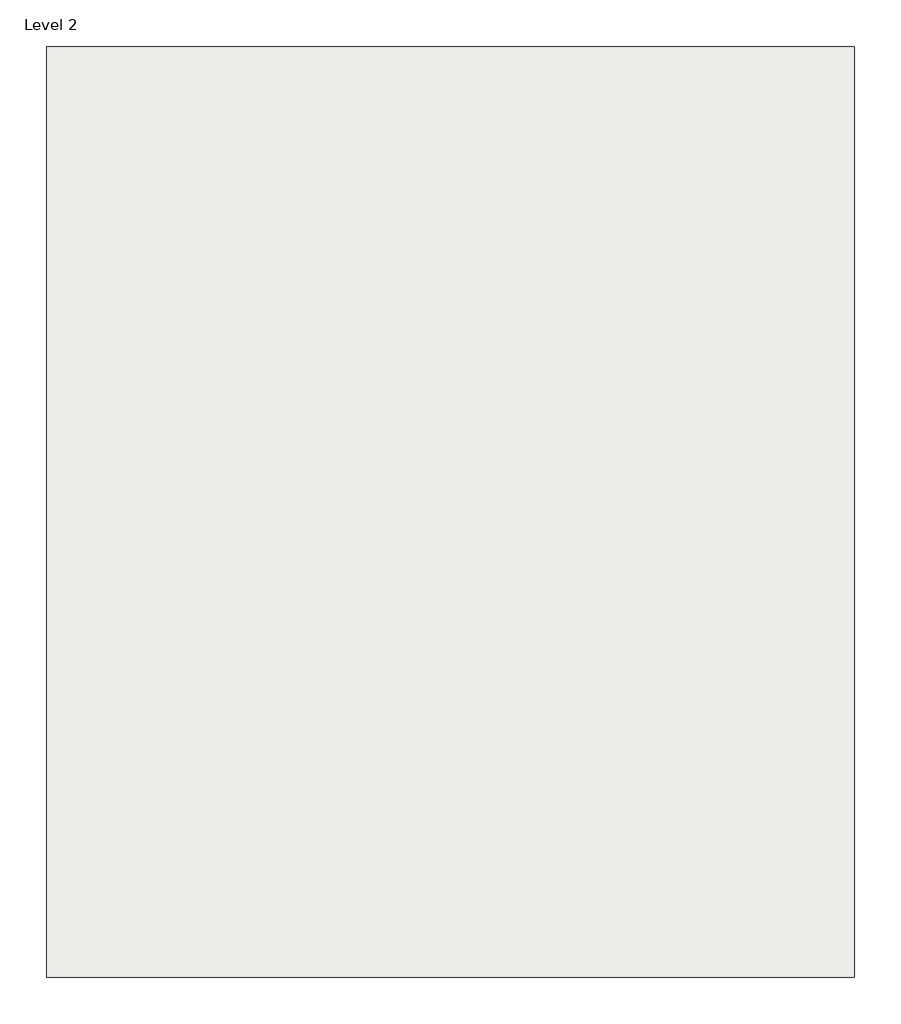
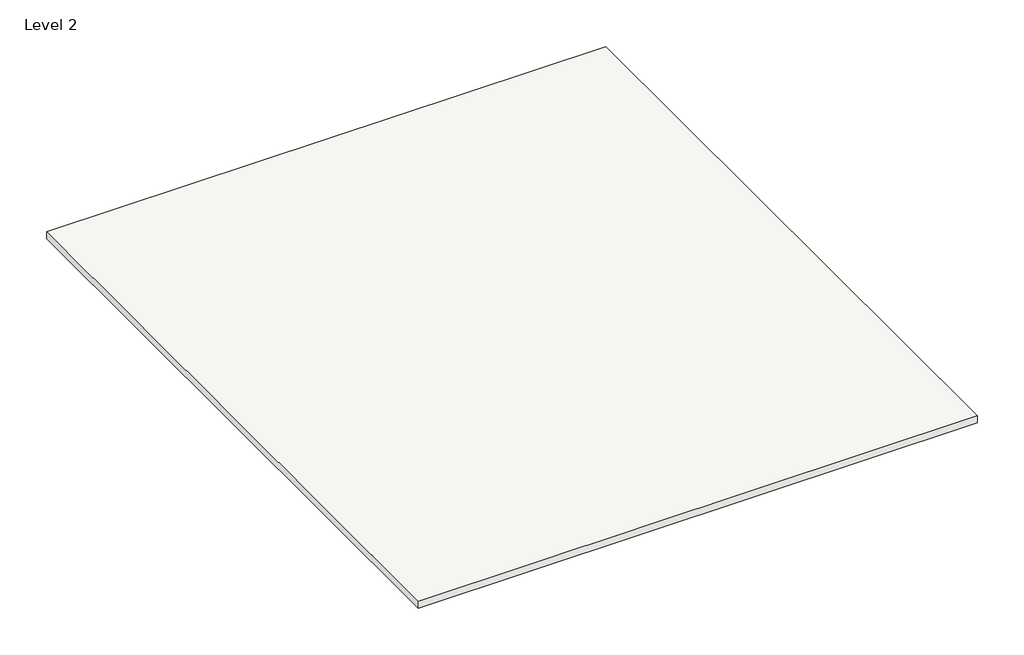
# One storey: 1 roof.
"""IFC4 building model written with IfcOpenShell, lengths in millimetres."""

from ifc_helpers import new_model, si_unit, frame, origin, place, context, project, spatial, polyline, outline, extrude, element, save

model = new_model("IFC4")

# Units and contexts
model_context = context("Model", 3, world=origin())
ifc_project = project(units=[si_unit("LENGTHUNIT", "METRE", prefix="MILLI")], contexts=[model_context])

# Site, building, storey
site = spatial("IfcSite", under=ifc_project)
building = spatial("IfcBuilding", under=site)
storey = spatial("IfcBuildingStorey", under=building, Name="Level 2", Elevation=3048.0)

# Roof
placement = place(None, origin())
element("IfcRoof", 1, ObjectType="Wood Rafter 8\" - Asphalt Shingle - Insulated", at=placement, inside=storey, context=model_context, shape_type="SweptSolid", body=[
    extrude(outline(polyline([(-17641.7484731, 12572.6442281), (-1588.9484731, 12572.6442281), (-1588.9484731, -5918.5557719), (-17641.7484731, -5918.5557719), (-17641.7484731, 12572.6442281)])), frame((0.0, 0.0, 3048.0), z_axis=(0.0, 0.0, 1.0), x_axis=(1.0, 0.0, 0.0)), (0.0, 0.0, 1.0), 212.725),
])

save(model, "model.ifc")

# Revit data of these elements
# Type "Wood Rafter 8\" - Asphalt Shingle - Insulated"
#   Assembly Code = "B1020"
#   Layers, outside or top first: 0' - 0 1/4" "Asphalt Shingle" (function 4); 0' - 0 5/8" "Plywood, Sheathing" (function 2); 0' - 7 1/2" "Structure, Wood Joist/Rafter Layer, Batt Insulation" (function 1)
# Element 1 (IfcRoof, "Wood Rafter 8\" - Asphalt Shingle - Insulated")
#   built-in parameter 1001705 = 10.6979 (stored number, unit not read)
#   built-in parameter 1001710 = 33615
#   Phase Created = New Construction
#   Materials on its faces: "Structure, Wood Joist/Rafter Layer, Batt Insulation", "Asphalt Shingle"
# Materials
#   "Asphalt Shingle": class "Generic", colour RGB 155 155 155, transparency 0, Description = "Asphalt roofing shingle", Cost = 0
#   "Plywood, Sheathing": class "Wood", colour RGB 212 179 113, transparency 0, Description = "Plywood, sheathing grade", Cost = 0
#   "Structure, Wood Joist/Rafter Layer, Batt Insulation": class "Wood", colour RGB 127 127 127, transparency 0, Description = "Wood framing, insulated", Cost = 0
